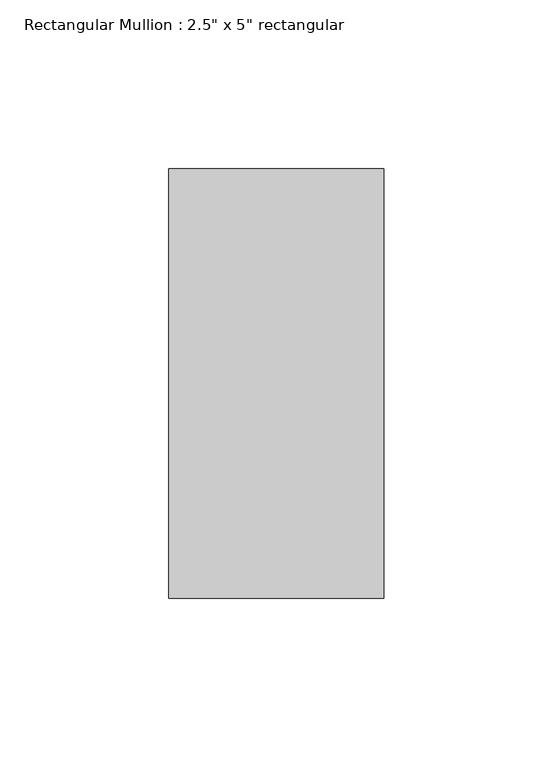
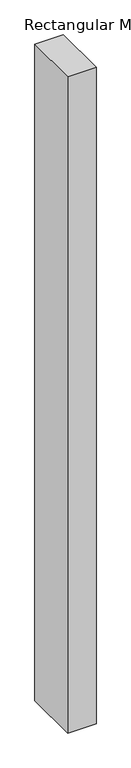
"""IFC4 building model written with IfcOpenShell, lengths in millimetres: member geometry."""

from ifc_helpers import new_model, si_unit, frame, origin, place, context, project, spatial, polyline, outline, extrude, source, transform, mapped, element, save


def member_3fd136ac(model_context):
    return source(origin(), model_context, "Body", "SweptSolid", [
        extrude(outline(polyline([(0.0, 63.5), (0.0, -63.5), (-63.5, -63.5), (-63.5, 63.5), (0.0, 63.5)])), frame((0.0, 0.0, -1553.5106693), z_axis=(0.0, 0.0, 1.0), x_axis=(1.0, 0.0, 0.0)), (0.0, 0.0, 1.0), 1553.5106693),
    ])


if __name__ == "__main__":
    model = new_model("IFC4")
    model_context = context("Model", 3, world=origin())
    ifc_project = project(units=[si_unit("LENGTHUNIT", "METRE", prefix="MILLI")], contexts=[model_context])
    site = spatial("IfcSite", under=ifc_project)
    building = spatial("IfcBuilding", under=site)
    placement = place(None, origin())
    member_shape = member_3fd136ac(model_context)
    element("IfcMember", 1, ObjectType="Rectangular Mullion : 2.5\" x 5\" rectangular", at=placement, inside=building, context=model_context, shape_type="MappedRepresentation", body=[
        mapped(member_shape, transform((0.0, 0.0, 0.0), x_axis=(1.0, 0.0, 0.0), y_axis=(0.0, 1.0, 0.0), z_axis=(0.0, 0.0, 1.0))),
    ])
    save(model, "model.ifc")

# Revit data of these elements
# Type "Rectangular Mullion : 2.5\" x 5\" rectangular"
#   built-in parameter 1007304 = 0.416667 (stored number, unit not read)
#   built-in parameter 1007301 = 0.104167 (stored number, unit not read)
#   built-in parameter 1007300 = 0.104167 (stored number, unit not read)
# Element 1 (IfcMember, "Rectangular Mullion : 2.5\" x 5\" rectangular")
#   Materials on its faces: "Aluminum"
# Materials
#   "Aluminum": class "Metal", colour RGB 247 247 247, transparency 0, Description = "Aluminum 6061", Cost = 0
